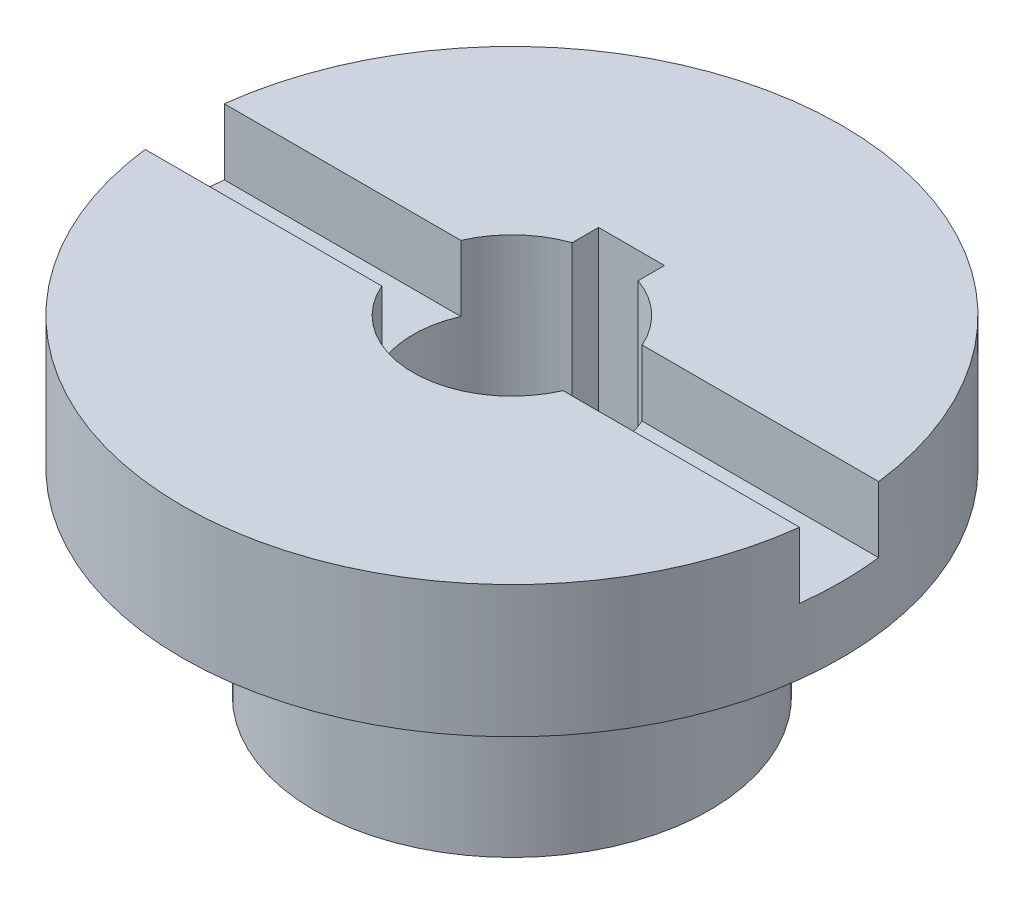
from build123d import *

# Parameters (mm, degrees)
BORE_KEYWAY_4MM_DEPTH  = 87.602540378
CROSS_SLOT_SKETCH_W    = 119.375340358
CROSS_SLOT_SKETCH_H    = 12
CROSS_SLOT_12X10_DEPTH = 10


with BuildPart() as part:
    # Flange Profile Sketch → Flange Body Revolve (revolve)
    with BuildSketch(Plane.XY, mode=Mode.PRIVATE) as flange_body_revolve_sk:
        with BuildLine():
            Line((0, 0), (50, 0))
            Line((50, 0), (50, -20))
            Line((50, -20), (33, -20))
            ThreePointArc((33, -20), (30.878679656, -20.878679656), (30, -23))
            Line((30, -23), (30, -50))
            Line((30, -50), (0, -50))
            Line((0, -50), (0, 0))
        make_face()
    revolve(flange_body_revolve_sk.sketch.rotate(Axis((0, 54.118773946, 0), (0, -1, 0)), 90), axis=Axis((0, 54.118773946, 0), (0, -1, 0)))

    # Bore Keyway Sketch → Bore Keyway 4mm (cut, through all)
    with BuildSketch(Plane(origin=(0, 0, 0), x_dir=(1, 0, 0), z_dir=(0, 1, 0))):
        with BuildLine():
            Line((-5, 14.142135624), (-5, 18.142135624))
            Line((-5, 18.142135624), (5, 18.142135624))
            Line((5, 18.142135624), (5, 14.142135624))
            ThreePointArc((5, 14.142135624), (0, -15), (-5, 14.142135624))
        make_face()
    extrude(amount=-BORE_KEYWAY_4MM_DEPTH, mode=Mode.SUBTRACT)

    # Cross Slot Sketch → Cross Slot 12x10 (cut)
    with BuildSketch(Plane(origin=(0, 0, 0), x_dir=(1, 0, 0), z_dir=(0, 1, 0))):
        Rectangle(CROSS_SLOT_SKETCH_W, CROSS_SLOT_SKETCH_H)
    extrude(amount=-CROSS_SLOT_12X10_DEPTH, mode=Mode.SUBTRACT)


solid = part.part
